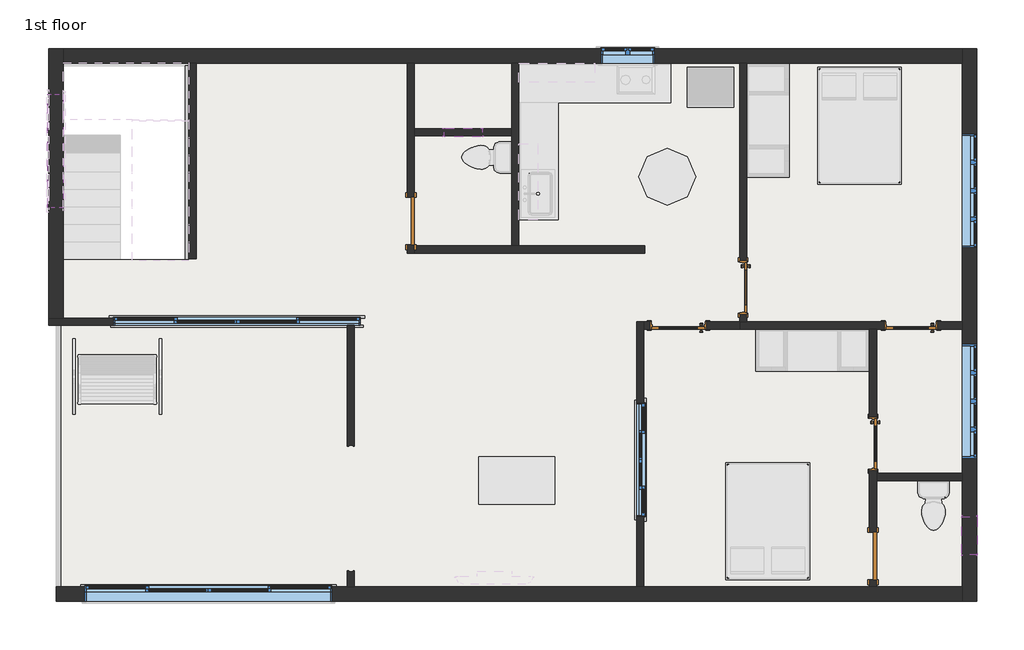
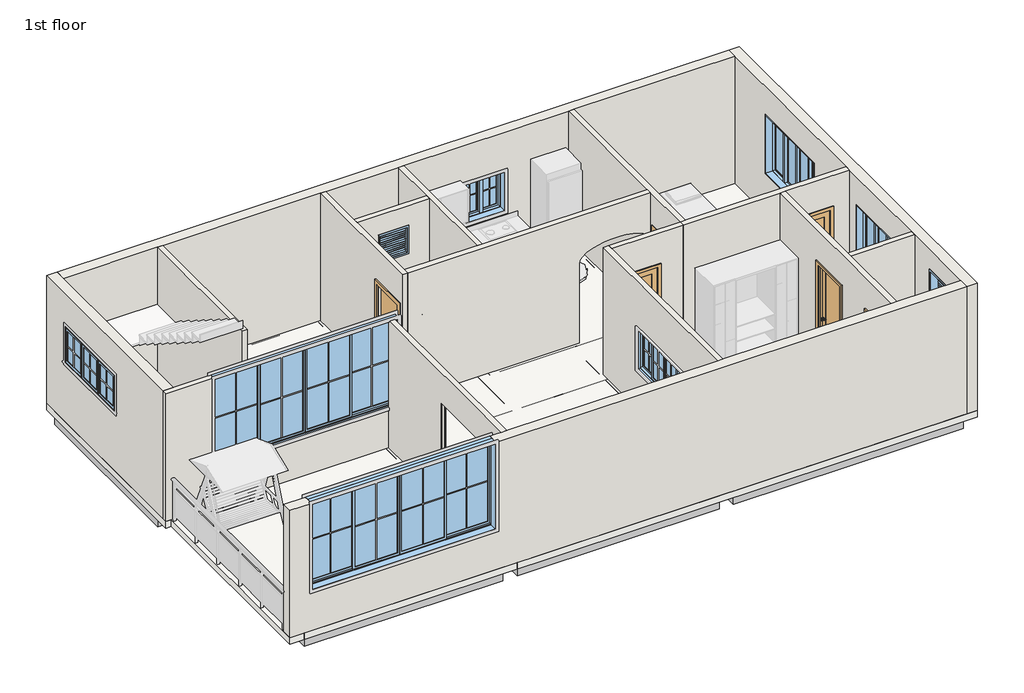
# One storey, part 1 of 2: 17 walls, 9 windows, 8 beams, 6 doors, 1 slab.
# Revit data of these elements (continued)
# Element 33 (IfcWindow, "Window-Awning-Triple-Horizontal : 72\" x 32\"") (continued)
#   Exterior Wall Closure = 0.104167 ft
#   Interior Trim Visibility = yes
#   Exterior Trim Visibility = yes
#   Phase Created = New Construction
#   Materials on its faces: "Wood - Stained", "Glass", "Clad - White"
# Element 34 (IfcWindow, "Window-Casement-Double : 34\" x 36\"")
#   Mark = "18"
#   Window Inset = 0 ft
#   Interior Wall Closure = 0.1875 ft
#   Frame Extension = 0.020833 ft
#   Exterior Wall Closure = 0.104167 ft
#   Interior Trim Visibility = yes
#   Exterior Trim Visibility = yes
#   Phase Created = New Construction
#   Materials on its faces: "Wood - Stained", "Glass", "Clad - White"
# Element 35 (IfcWindow, "Window-Casement-Multi-Sash-Horizontal : 72\" x 53\"")
#   Mark = "13"
#   Window Inset = 0.052083 ft
#   Frame Gap 3 = 0.13737 ft
#   Frame Gap 2 = 0.052083 ft
#   Phase Created = New Construction
#   Materials on its faces: "Metal - Aluminum", "Glass"
# Element 36 (IfcWindow, "Window-Casement-Multi-Sash-Horizontal : 72\" x 53\"")
#   Mark = "16"
#   Window Inset = 0.052083 ft
#   Frame Gap 3 = 0.13737 ft
#   Frame Gap 2 = 0.052083 ft
#   Phase Created = New Construction
#   Materials on its faces: "Metal - Aluminum", "Glass"
# Element 37 (IfcWindow, "Window-Louvers : 24\" x 24\"")
#   Mark = "14"
#   Blade Width = 1.875 ft
#   Phase Created = New Construction
#   Materials on its faces: "Birch"
# Element 38 (IfcWindow, "Window-Louvers : 24\" x 24\"")
#   Mark = "15"
#   Blade Width = 1.875 ft
#   Phase Created = New Construction
#   Materials on its faces: "Birch"
# Element 39 (IfcWindow, "Window-Sliding-Four : 156\" x 78\"")
#   Mark = "11"
#   Window Inset = 0 ft
#   Interior Wall Closure = 0.216146 ft
#   Frame Extension = 0.020833 ft
#   Exterior Wall Closure = 0.104167 ft
#   Interior Trim Visibility = yes
#   Indicator Visibility = yes
#   Exterior Trim Visibility = yes
#   Phase Created = New Construction
#   Materials on its faces: "Wood - Stained", "Glass", "Clad - White"
# Element 40 (IfcWindow, "Window-Sliding-Four : 180\" x 78\"")
#   Mark = "28"
#   Window Inset = 0 ft
#   Interior Wall Closure = 0.216146 ft
#   Frame Extension = 0.020833 ft
#   Exterior Wall Closure = 0.104167 ft
#   Interior Trim Visibility = yes
#   Indicator Visibility = yes
#   Exterior Trim Visibility = yes
#   Phase Created = New Construction
#   Materials on its faces: "Wood - Stained", "Glass", "Clad - White"
# Element 41 (IfcWindow, "Window-Sliding-Four : 72\" x 36\"")
#   Mark = "12"
#   Window Inset = 0 ft
#   Interior Wall Closure = 0.216146 ft
#   Frame Extension = 0.020833 ft
#   Exterior Wall Closure = 0.104167 ft
#   Interior Trim Visibility = yes
#   Indicator Visibility = yes
#   Exterior Trim Visibility = yes
#   Phase Created = New Construction
#   Materials on its faces: "Wood - Stained", "Glass", "Clad - White"
# Materials
#   "Concrete, Cast-in-Place gray": class "Concrete", colour RGB 192 192 192, transparency 0, Description = "Cast-in-place concrete", Cost = 0
#   "Cherry": class "Wood", colour RGB 226 177 128, transparency 0, Description = "Prunus Serotina", Cost = 0
#   "Aluminum": class "Metal", colour RGB 247 247 247, transparency 0, Description = "Aluminum 6061", Cost = 0
#   "Door - Panel": class "Wood", colour RGB 210 159 95, transparency 0, Cost = 0
#   "Door - Frame": colour RGB 118 70 51, transparency 0, Cost = 0
#   "Wood - Stained": class "Wood", colour RGB 224 178 126, transparency 0, Cost = 0
#   "Glass": class "Glass", colour RGB 0 128 192, transparency 0.75, Description = "Soda Lime Glass", Cost = 0
#   "Clad - White": class "Wood", colour RGB 242 242 238, transparency 0, Cost = 0
#   "Metal - Aluminum": class "Metal", colour RGB 247 247 247, transparency 0
#   "Birch": class "Wood", colour RGB 224 178 126, transparency 0, Description = "Betula Alleghaniensis", Cost = 0
#   "Default Floor": colour RGB 128 128 128, transparency 0, Cost = 0
#   "Default Wall": colour RGB 128 128 128, transparency 0, Cost = 0
